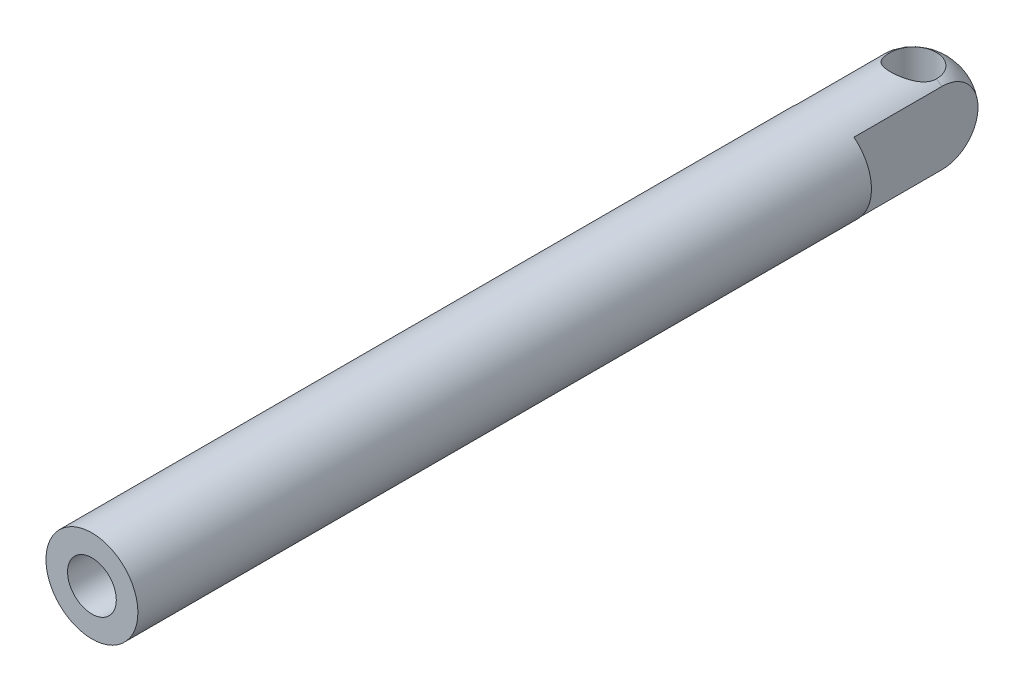
ISO-10303-21;
HEADER;
FILE_DESCRIPTION(('STEP AP214'),'2;1');
FILE_NAME('part.step','',(''),(''),'','','');
FILE_SCHEMA(('AUTOMOTIVE_DESIGN { 1 0 10303 214 1 1 1 1 }'));
ENDSEC;
DATA;
#1=APPLICATION_CONTEXT('core data for automotive mechanical design processes');
#2=APPLICATION_PROTOCOL_DEFINITION('international standard','automotive_design',2000,#1);
#3=PRODUCT_CONTEXT('',#1,'mechanical');
#4=PRODUCT('Part','Part','',(#3));
#5=PRODUCT_RELATED_PRODUCT_CATEGORY('part','',(#4));
#6=PRODUCT_DEFINITION_FORMATION('','',#4);
#7=PRODUCT_DEFINITION_CONTEXT('part definition',#1,'design');
#8=PRODUCT_DEFINITION('design','',#6,#7);
#9=PRODUCT_DEFINITION_SHAPE('','',#8);
#10=(LENGTH_UNIT() NAMED_UNIT(*) SI_UNIT(.MILLI.,.METRE.));
#11=(NAMED_UNIT(*) PLANE_ANGLE_UNIT() SI_UNIT($,.RADIAN.));
#12=(NAMED_UNIT(*) SI_UNIT($,.STERADIAN.) SOLID_ANGLE_UNIT());
#13=UNCERTAINTY_MEASURE_WITH_UNIT(LENGTH_MEASURE(1.E-05),#10,'distance_accuracy_value','');
#14=(GEOMETRIC_REPRESENTATION_CONTEXT(3) GLOBAL_UNCERTAINTY_ASSIGNED_CONTEXT((#13)) GLOBAL_UNIT_ASSIGNED_CONTEXT((#10,
#11,#12)) REPRESENTATION_CONTEXT('',''));
#15=CARTESIAN_POINT('',(0.,0.,0.));
#16=DIRECTION('',(0.,0.,1.));
#17=DIRECTION('',(1.,0.,0.));
#18=AXIS2_PLACEMENT_3D('',#15,#16,#17);
#19=CARTESIAN_POINT('',(0.,0.,1100.));
#20=DIRECTION('',(0.,0.,-1.));
#21=DIRECTION('',(-1.,0.,0.));
#22=AXIS2_PLACEMENT_3D('',#19,#20,#21);
#23=CYLINDRICAL_SURFACE('',#22,115.);
#24=CARTESIAN_POINT('',(0.,0.,1100.));
#25=DIRECTION('',(0.,0.,1.));
#26=DIRECTION('',(1.,0.,0.));
#27=AXIS2_PLACEMENT_3D('',#24,#25,#26);
#28=CIRCLE('',#27,115.);
#29=CARTESIAN_POINT('',(115.,0.,1100.));
#30=VERTEX_POINT('',#29);
#31=EDGE_CURVE('E116',#30,#30,#28,.T.);
#32=ORIENTED_EDGE('',*,*,#31,.F.);
#33=EDGE_LOOP('',(#32));
#34=FACE_BOUND('',#33,.T.);
#35=CARTESIAN_POINT('',(0.,0.,-955.));
#36=DIRECTION('',(0.,0.,-1.));
#37=DIRECTION('',(-1.,0.,0.));
#38=AXIS2_PLACEMENT_3D('',#35,#36,#37);
#39=CIRCLE('',#38,115.);
#40=CARTESIAN_POINT('',(-71.25,90.2686961244041,-955.));
#41=VERTEX_POINT('',#40);
#42=CARTESIAN_POINT('',(-57.5,99.5929214352104,-955.));
#43=VERTEX_POINT('',#42);
#44=EDGE_CURVE('E94',#41,#43,#39,.T.);
#45=ORIENTED_EDGE('',*,*,#44,.F.);
#46=DIRECTION('',(0.,0.,-1.));
#47=VECTOR('',#46,1.);
#48=CARTESIAN_POINT('',(-71.2499999999997,90.2686961244043,1100.));
#49=LINE('',#48,#47);
#50=CARTESIAN_POINT('',(-71.25,90.2686961244041,-735.));
#51=VERTEX_POINT('',#50);
#52=EDGE_CURVE('E64',#41,#51,#49,.F.);
#53=ORIENTED_EDGE('',*,*,#52,.T.);
#54=CARTESIAN_POINT('',(0.,0.,-735.));
#55=DIRECTION('',(0.,0.,1.));
#56=DIRECTION('',(1.,0.,0.));
#57=AXIS2_PLACEMENT_3D('',#54,#55,#56);
#58=CIRCLE('',#57,115.);
#59=CARTESIAN_POINT('',(-71.25,-90.2686961244041,-735.));
#60=VERTEX_POINT('',#59);
#61=EDGE_CURVE('E49',#51,#60,#58,.T.);
#62=ORIENTED_EDGE('',*,*,#61,.T.);
#63=DIRECTION('',(0.,0.,-1.));
#64=VECTOR('',#63,1.);
#65=CARTESIAN_POINT('',(-71.2499999999997,-90.2686961244043,1100.));
#66=LINE('',#65,#64);
#67=CARTESIAN_POINT('',(-71.2499999999997,-90.2686961244043,-955.));
#68=VERTEX_POINT('',#67);
#69=EDGE_CURVE('E108',#60,#68,#66,.T.);
#70=ORIENTED_EDGE('',*,*,#69,.T.);
#71=CARTESIAN_POINT('',(-57.5,-99.5929214352104,-955.));
#72=VERTEX_POINT('',#71);
#73=EDGE_CURVE('E57',#72,#68,#39,.T.);
#74=ORIENTED_EDGE('',*,*,#73,.F.);
#75=CARTESIAN_POINT('',(0.,-115.,-897.5));
#76=CARTESIAN_POINT('',(0.756039926193434,-114.999999631967,-897.500000432809));
#77=CARTESIAN_POINT('',(1.51209474049783,-114.9925400002,-897.514915561743));
#78=CARTESIAN_POINT('',(3.02281407863114,-114.962748266929,-897.57453400003));
#79=CARTESIAN_POINT('',(3.77747843127836,-114.940414442841,-897.619240759561));
#80=CARTESIAN_POINT('',(5.28412678755319,-114.881010387195,-897.7383268216));
#81=CARTESIAN_POINT('',(6.03610984888096,-114.84393540827,-897.812715683214));
#82=CARTESIAN_POINT('',(7.53579035985064,-114.755288294118,-897.990946701532));
#83=CARTESIAN_POINT('',(8.28348735976146,-114.703714664983,-898.094791893359));
#84=CARTESIAN_POINT('',(9.77431659971768,-114.586310667988,-898.331814579295));
#85=CARTESIAN_POINT('',(10.5174397895978,-114.520457961659,-898.46503803896));
#86=CARTESIAN_POINT('',(11.9965952698237,-114.374972804063,-898.760327289052));
#87=CARTESIAN_POINT('',(12.732626832776,-114.295338954809,-898.922396005651));
#88=CARTESIAN_POINT('',(14.9278119005363,-114.036525121805,-899.451152414411));
#89=CARTESIAN_POINT('',(16.374630682964,-113.837387021987,-899.860482083411));
#90=CARTESIAN_POINT('',(19.2192553604664,-113.391738083302,-900.786533039665));
#91=CARTESIAN_POINT('',(20.6172308265571,-113.145415580846,-901.302828021905));
#92=CARTESIAN_POINT('',(23.3621431455185,-112.610679940459,-902.438926815576));
#93=CARTESIAN_POINT('',(24.7090788987355,-112.322265896311,-903.058732855606));
#94=CARTESIAN_POINT('',(27.3444469912767,-111.709942598463,-904.396494277195));
#95=CARTESIAN_POINT('',(28.6328903145282,-111.386040048249,-905.114431128975));
#96=CARTESIAN_POINT('',(31.1454916920329,-110.709761453484,-906.6432915934));
#97=CARTESIAN_POINT('',(32.3696474551825,-110.357384395282,-907.454218516786));
#98=CARTESIAN_POINT('',(34.8203558940024,-109.609679277469,-909.215661471305));
#99=CARTESIAN_POINT('',(36.0425740731368,-109.213042473018,-910.171654104824));
#100=CARTESIAN_POINT('',(38.4031684838954,-108.405503186936,-912.176583704386));
#101=CARTESIAN_POINT('',(39.5415418254895,-107.994600214285,-913.225523871476));
#102=CARTESIAN_POINT('',(41.7300653973575,-107.167956612408,-915.411549309096));
#103=CARTESIAN_POINT('',(42.7801526952142,-106.752212768839,-916.54869636393));
#104=CARTESIAN_POINT('',(44.7862205870241,-105.926254101274,-918.905141627569));
#105=CARTESIAN_POINT('',(45.7421970798222,-105.516039518904,-920.124443412612));
#106=CARTESIAN_POINT('',(47.625340381661,-104.680318438948,-922.737508610054));
#107=CARTESIAN_POINT('',(48.544498522214,-104.256099974802,-924.137466526771));
#108=CARTESIAN_POINT('',(50.2609148362852,-103.43956750798,-927.019604493645));
#109=CARTESIAN_POINT('',(51.0581648876982,-103.047255631889,-928.501790013246));
#110=CARTESIAN_POINT('',(52.1567191513199,-102.493144746503,-930.779400826146));
#111=CARTESIAN_POINT('',(52.5066497716825,-102.31418552947,-931.547570106338));
#112=CARTESIAN_POINT('',(53.1732926756907,-101.969317877728,-933.101026779879));
#113=CARTESIAN_POINT('',(53.490008967781,-101.80340786879,-933.886312093745));
#114=CARTESIAN_POINT('',(54.0893246377893,-101.486254881608,-935.472735887457));
#115=CARTESIAN_POINT('',(54.3719226434949,-101.335012493333,-936.273875003424));
#116=CARTESIAN_POINT('',(54.9020568842566,-101.04877489629,-937.890424944825));
#117=CARTESIAN_POINT('',(55.1495979508498,-100.913777449036,-938.705833786171));
#118=CARTESIAN_POINT('',(55.5950926584644,-100.668994003689,-940.300358924188));
#119=CARTESIAN_POINT('',(55.7951236206591,-100.558184383544,-941.078738099718));
#120=CARTESIAN_POINT('',(56.1627635665738,-100.353317269723,-942.645198713617));
#121=CARTESIAN_POINT('',(56.3303768728474,-100.259257542757,-943.433278843539));
#122=CARTESIAN_POINT('',(56.6326291042369,-100.088837733909,-945.017723949384));
#123=CARTESIAN_POINT('',(56.7672647241471,-100.012479426202,-945.814089747411));
#124=CARTESIAN_POINT('',(57.0030171865704,-99.8782981348512,-947.413225495293));
#125=CARTESIAN_POINT('',(57.1041380984085,-99.8204729009671,-948.215994655528));
#126=CARTESIAN_POINT('',(57.2724234473565,-99.7240137904763,-949.825653897568));
#127=CARTESIAN_POINT('',(57.3396121667856,-99.6853661904514,-950.632540613923));
#128=CARTESIAN_POINT('',(57.439863213353,-99.6276339662686,-952.249030383599));
#129=CARTESIAN_POINT('',(57.4729296704659,-99.6085469746021,-953.058633096288));
#130=CARTESIAN_POINT('',(57.504809509286,-99.5901465279169,-954.678737213077));
#131=CARTESIAN_POINT('',(57.5036235394099,-99.5908326985817,-955.489238599875));
#132=CARTESIAN_POINT('',(57.4670182378401,-99.6119572651791,-957.109131910917));
#133=CARTESIAN_POINT('',(57.4315998689858,-99.6323951055655,-957.918523865724));
#134=CARTESIAN_POINT('',(57.2867443378253,-99.7158050688549,-960.148629469244));
#135=CARTESIAN_POINT('',(57.1415111568199,-99.7992980006931,-961.566461654727));
#136=CARTESIAN_POINT('',(56.74715307412,-100.024054388127,-964.382587204817));
#137=CARTESIAN_POINT('',(56.4980379217935,-100.165312422419,-965.780882390256));
#138=CARTESIAN_POINT('',(55.8987313897626,-100.500993289944,-968.549474129445));
#139=CARTESIAN_POINT('',(55.5485146876636,-100.695429441789,-969.919763576555));
#140=CARTESIAN_POINT('',(54.7506543690294,-101.131460009223,-972.623950185859));
#141=CARTESIAN_POINT('',(54.3030055628721,-101.373056936711,-973.957845405292));
#142=CARTESIAN_POINT('',(53.3028640421449,-101.902561337218,-976.612807639544));
#143=CARTESIAN_POINT('',(52.7481799858778,-102.191413138314,-977.932859168227));
#144=CARTESIAN_POINT('',(51.5455433044256,-102.803267968911,-980.521441799243));
#145=CARTESIAN_POINT('',(50.8975906337853,-103.126271015054,-981.789972876468));
#146=CARTESIAN_POINT('',(49.5125582915078,-103.798357758824,-984.270726308318));
#147=CARTESIAN_POINT('',(48.7754481390498,-104.147450360174,-985.482929208521));
#148=CARTESIAN_POINT('',(47.2164488041148,-104.863448210345,-987.846019316552));
#149=CARTESIAN_POINT('',(46.3945539489378,-105.230354650168,-988.996902413826));
#150=CARTESIAN_POINT('',(44.5604896200246,-106.021140402594,-991.375052976015));
#151=CARTESIAN_POINT('',(43.5374093623827,-106.446341862118,-992.593485064299));
#152=CARTESIAN_POINT('',(41.3940851145652,-107.297994310601,-994.94128936598));
#153=CARTESIAN_POINT('',(40.2738339511412,-107.724445389559,-996.070654992638));
#154=CARTESIAN_POINT('',(37.9411110892785,-108.568001016734,-998.234874912984));
#155=CARTESIAN_POINT('',(36.7285966602381,-108.985101116957,-999.269684920083));
#156=CARTESIAN_POINT('',(34.2176012597706,-109.799352171425,-1001.23797774279));
#157=CARTESIAN_POINT('',(32.9191196677261,-110.196502981613,-1002.17145982675));
#158=CARTESIAN_POINT('',(30.180184047429,-110.978726236119,-1003.97157632688));
#159=CARTESIAN_POINT('',(28.7359340199946,-111.362373826484,-1004.83306989169));
#160=CARTESIAN_POINT('',(25.7687974093903,-112.086130871539,-1006.4301230848));
#161=CARTESIAN_POINT('',(24.2459071685366,-112.426238298542,-1007.16567684854));
#162=CARTESIAN_POINT('',(21.1327463003638,-113.052758086648,-1008.50256724992));
#163=CARTESIAN_POINT('',(19.5425192850707,-113.339204569421,-1009.10398922533));
#164=CARTESIAN_POINT('',(16.3059802117296,-113.849890864604,-1010.16579197716));
#165=CARTESIAN_POINT('',(14.659674629808,-114.074137832845,-1010.62618897864));
#166=CARTESIAN_POINT('',(11.4632047192093,-114.437600072419,-1011.36762870229));
#167=CARTESIAN_POINT('',(9.91637286310852,-114.582320238039,-1011.66036914825));
#168=CARTESIAN_POINT('',(6.79940917810755,-114.809446464326,-1012.11828715779));
#169=CARTESIAN_POINT('',(5.22927862129342,-114.891855914424,-1012.28347165986));
#170=CARTESIAN_POINT('',(2.07932335511353,-114.99199375301,-1012.48405134883));
#171=CARTESIAN_POINT('',(0.499502774961316,-115.009748002694,-1012.51949842896));
#172=CARTESIAN_POINT('',(-2.65704791013921,-114.980132207341,-1012.46026065505));
#173=CARTESIAN_POINT('',(-4.23377814876672,-114.932765044441,-1012.36558156011));
#174=CARTESIAN_POINT('',(-7.24900068560403,-114.780448517955,-1012.05976820056));
#175=CARTESIAN_POINT('',(-8.68872217543315,-114.680254828179,-1011.8582451553));
#176=CARTESIAN_POINT('',(-11.5442945106091,-114.428071157171,-1011.34787232871));
#177=CARTESIAN_POINT('',(-12.9601468857035,-114.276084508642,-1011.03902945303));
#178=CARTESIAN_POINT('',(-15.7589346501385,-113.923859304687,-1010.31722028618));
#179=CARTESIAN_POINT('',(-17.1418682040933,-113.723618065721,-1009.90424820412));
#180=CARTESIAN_POINT('',(-19.86654595913,-113.279415572935,-1008.97815295026));
#181=CARTESIAN_POINT('',(-21.2082884268221,-113.035452482172,-1008.46502557044));
#182=CARTESIAN_POINT('',(-23.880897489362,-112.5016105184,-1007.32706764311));
#183=CARTESIAN_POINT('',(-25.2103616515162,-112.210620237904,-1006.69946785276));
#184=CARTESIAN_POINT('',(-27.8111662225543,-111.59446813568,-1005.34815623474));
#185=CARTESIAN_POINT('',(-29.082506120613,-111.269306013714,-1004.62444356261));
#186=CARTESIAN_POINT('',(-31.5616183205955,-110.591664351637,-1003.0857921916));
#187=CARTESIAN_POINT('',(-32.7693696687149,-110.239175900343,-1002.27082369515));
#188=CARTESIAN_POINT('',(-35.1158123979574,-109.514327042851,-1000.55483038709));
#189=CARTESIAN_POINT('',(-36.2544999782216,-109.141965545075,-999.653800846205));
#190=CARTESIAN_POINT('',(-38.5665301149181,-108.347865372805,-997.677944661801));
#191=CARTESIAN_POINT('',(-39.7322855784827,-107.924869834846,-996.594740149521));
#192=CARTESIAN_POINT('',(-41.9695388226546,-107.074692698471,-994.336167972647));
#193=CARTESIAN_POINT('',(-43.0410307794307,-106.647510843224,-993.160794622108));
#194=CARTESIAN_POINT('',(-44.5734979250476,-106.011838231184,-991.332993713112));
#195=CARTESIAN_POINT('',(-45.0720701748748,-105.800701644033,-990.712636948676));
#196=CARTESIAN_POINT('',(-46.04350748944,-105.381569171776,-989.451110862577));
#197=CARTESIAN_POINT('',(-46.5163747063028,-105.173573024797,-988.809943290476));
#198=CARTESIAN_POINT('',(-47.4356642828128,-104.762165642518,-987.507583576832));
#199=CARTESIAN_POINT('',(-47.8820891385812,-104.558753975576,-986.846393334334));
#200=CARTESIAN_POINT('',(-48.7479330302106,-104.157893217983,-985.504539423803));
#201=CARTESIAN_POINT('',(-49.1673432718118,-103.960446080004,-984.823869517525));
#202=CARTESIAN_POINT('',(-50.4230543067088,-103.360550292388,-982.687193445124));
#203=CARTESIAN_POINT('',(-51.2121770973233,-102.970727111135,-981.199460793565));
#204=CARTESIAN_POINT('',(-52.6604836742353,-102.237631258297,-978.151023950491));
#205=CARTESIAN_POINT('',(-53.3196816844298,-101.894353492302,-976.590327770044));
#206=CARTESIAN_POINT('',(-54.2051804569244,-101.424403053757,-974.203349911754));
#207=CARTESIAN_POINT('',(-54.4830649598738,-101.275283870952,-973.400273678963));
#208=CARTESIAN_POINT('',(-55.0036483734081,-100.993496724154,-971.780112954271));
#209=CARTESIAN_POINT('',(-55.2463563693533,-100.860824513534,-970.963032140649));
#210=CARTESIAN_POINT('',(-55.6957760306153,-100.613350653786,-969.316387578991));
#211=CARTESIAN_POINT('',(-55.9024885524288,-100.498548579451,-968.486824128485));
#212=CARTESIAN_POINT('',(-56.2791501611203,-100.288104202955,-966.816929259857));
#213=CARTESIAN_POINT('',(-56.4490977748551,-100.192462668553,-965.976597411681));
#214=CARTESIAN_POINT('',(-56.736992902327,-100.029686864408,-964.368319865377));
#215=CARTESIAN_POINT('',(-56.8583669988458,-99.9606969052523,-963.601173319719));
#216=CARTESIAN_POINT('',(-57.070067628939,-99.8399832319084,-962.061258907232));
#217=CARTESIAN_POINT('',(-57.1603946750298,-99.7882592326992,-961.288491133412));
#218=CARTESIAN_POINT('',(-57.3096654456911,-99.7026060629048,-959.738989810187));
#219=CARTESIAN_POINT('',(-57.3686109205854,-99.6686758998606,-958.962256484403));
#220=CARTESIAN_POINT('',(-57.454904088652,-99.6189564332258,-957.406448322968));
#221=CARTESIAN_POINT('',(-57.4822515239774,-99.6031672776699,-956.627373468262));
#222=CARTESIAN_POINT('',(-57.5052371157365,-99.589898506077,-955.068933240547));
#223=CARTESIAN_POINT('',(-57.5008888683154,-99.5924110393675,-954.289568135489));
#224=CARTESIAN_POINT('',(-57.4605309260017,-99.615701142035,-952.731848495079));
#225=CARTESIAN_POINT('',(-57.4245176841276,-99.6364807576149,-951.953494082725));
#226=CARTESIAN_POINT('',(-57.3209665603307,-99.6960902023079,-950.399686608433));
#227=CARTESIAN_POINT('',(-57.2534334295366,-99.7349173110409,-949.624233126978));
#228=CARTESIAN_POINT('',(-57.0871056332497,-99.8302127262599,-948.077753745496));
#229=CARTESIAN_POINT('',(-56.9883079687483,-99.88668272511,-947.306728277448));
#230=CARTESIAN_POINT('',(-56.6673584968348,-100.069317044624,-945.149537369074));
#231=CARTESIAN_POINT('',(-56.410056996097,-100.214915854682,-943.770043780577));
#232=CARTESIAN_POINT('',(-55.7971757470509,-100.557435130884,-941.039939943489));
#233=CARTESIAN_POINT('',(-55.4416038290174,-100.75435150793,-939.689327402863));
#234=CARTESIAN_POINT('',(-54.635622638641,-101.193672037181,-937.023975355456));
#235=CARTESIAN_POINT('',(-54.1851912494906,-101.436086796053,-935.709244295455));
#236=CARTESIAN_POINT('',(-53.1934565263105,-101.959650626916,-933.122491205063));
#237=CARTESIAN_POINT('',(-52.652147181976,-102.240802260589,-931.850472006147));
#238=CARTESIAN_POINT('',(-51.4434079175519,-102.854583657747,-929.270862259647));
#239=CARTESIAN_POINT('',(-50.7699503776319,-103.189402290082,-927.966617402513));
#240=CARTESIAN_POINT('',(-49.3289391664945,-103.885976043569,-925.418788082898));
#241=CARTESIAN_POINT('',(-48.5613827724136,-104.247731944064,-924.175205377207));
#242=CARTESIAN_POINT('',(-46.9363907051099,-104.989394926069,-921.753152991897));
#243=CARTESIAN_POINT('',(-46.0789170228177,-105.369309646293,-920.574711172128));
#244=CARTESIAN_POINT('',(-44.2786768209794,-106.138385804183,-918.288060636244));
#245=CARTESIAN_POINT('',(-43.3359053699268,-106.52754777552,-917.179855987211));
#246=CARTESIAN_POINT('',(-41.2495738637216,-107.353992236728,-914.907834796143));
#247=CARTESIAN_POINT('',(-40.0955388897124,-107.791370788718,-913.75364709984));
#248=CARTESIAN_POINT('',(-37.6912537470597,-108.655423808158,-911.54561564665));
#249=CARTESIAN_POINT('',(-36.4409953740853,-109.082097358743,-910.491780463334));
#250=CARTESIAN_POINT('',(-33.8498872386978,-109.913774342929,-908.490683738797));
#251=CARTESIAN_POINT('',(-32.5089843692621,-110.318764819417,-907.543485555768));
#252=CARTESIAN_POINT('',(-29.7440808072623,-111.09613051583,-905.763412951452));
#253=CARTESIAN_POINT('',(-28.320084909544,-111.4685076146,-904.930531942821));
#254=CARTESIAN_POINT('',(-26.1232440513399,-111.996205177372,-903.769936298879));
#255=CARTESIAN_POINT('',(-25.3779570185928,-112.167534384552,-903.396646811582));
#256=CARTESIAN_POINT('',(-23.8696910734563,-112.498148703657,-902.681896513355));
#257=CARTESIAN_POINT('',(-23.1067141645341,-112.65743517086,-902.34043211985));
#258=CARTESIAN_POINT('',(-21.5641379346627,-112.962854193443,-901.690162046069));
#259=CARTESIAN_POINT('',(-20.7845340924405,-113.108983113067,-901.381365388595));
#260=CARTESIAN_POINT('',(-19.2104018054201,-113.386944229012,-900.797462745457));
#261=CARTESIAN_POINT('',(-18.4158751769259,-113.518778152167,-900.52235268994));
#262=CARTESIAN_POINT('',(-16.8152520483828,-113.766874008643,-900.007250953597));
#263=CARTESIAN_POINT('',(-16.0091876147387,-113.883172285347,-899.767177184207));
#264=CARTESIAN_POINT('',(-14.3853796211442,-114.099656635082,-899.322181835947));
#265=CARTESIAN_POINT('',(-13.5676375510337,-114.199844743814,-899.11725581555));
#266=CARTESIAN_POINT('',(-11.9225041939606,-114.383296966167,-898.74331011255));
#267=CARTESIAN_POINT('',(-11.0951175049056,-114.466568821348,-898.574274003672));
#268=CARTESIAN_POINT('',(-9.43227655563561,-114.615569489628,-898.272616922289));
#269=CARTESIAN_POINT('',(-8.59682357872582,-114.681301047154,-898.139990252923));
#270=CARTESIAN_POINT('',(-7.11657618506717,-114.78139287965,-897.938420570041));
#271=CARTESIAN_POINT('',(-6.47306173023466,-114.819495250392,-897.861836569897));
#272=CARTESIAN_POINT('',(-5.18343427575204,-114.884936794181,-897.730444717982));
#273=CARTESIAN_POINT('',(-4.53732203061077,-114.912278892345,-897.675630948065));
#274=CARTESIAN_POINT('',(-3.24322242753817,-114.956081540322,-897.587874735845));
#275=CARTESIAN_POINT('',(-2.59523500121499,-114.972541688093,-897.554933101627));
#276=CARTESIAN_POINT('',(-1.2981688664785,-114.994502486418,-897.510992723836));
#277=CARTESIAN_POINT('',(-0.649089920174928,-115.000000315971,-897.499999628416));
#278=CARTESIAN_POINT('',(0.,-115.,-897.5));
#279=B_SPLINE_CURVE_WITH_KNOTS('',3,(#75,#76,#77,#78,#79,#80,#81,#82,#83,#84,#85,#86,#87,#88,
#89,#90,#91,#92,#93,#94,#95,#96,#97,#98,#99,#100,#101,#102,#103,#104,#105,#106,#107,#108,#109,
#110,#111,#112,#113,#114,#115,#116,#117,#118,#119,#120,#121,#122,#123,#124,#125,#126,#127,#128,
#129,#130,#131,#132,#133,#134,#135,#136,#137,#138,#139,#140,#141,#142,#143,#144,#145,#146,#147,
#148,#149,#150,#151,#152,#153,#154,#155,#156,#157,#158,#159,#160,#161,#162,#163,#164,#165,#166,
#167,#168,#169,#170,#171,#172,#173,#174,#175,#176,#177,#178,#179,#180,#181,#182,#183,#184,#185,
#186,#187,#188,#189,#190,#191,#192,#193,#194,#195,#196,#197,#198,#199,#200,#201,#202,#203,#204,
#205,#206,#207,#208,#209,#210,#211,#212,#213,#214,#215,#216,#217,#218,#219,#220,#221,#222,#223,
#224,#225,#226,#227,#228,#229,#230,#231,#232,#233,#234,#235,#236,#237,#238,#239,#240,#241,#242,
#243,#244,#245,#246,#247,#248,#249,#250,#251,#252,#253,#254,#255,#256,#257,#258,#259,#260,#261,
#262,#263,#264,#265,#266,#267,#268,#269,#270,#271,#272,#273,#274,#275,#276,#277,#278),
.UNSPECIFIED.,.T.,.F.,(4,2,2,2,2,2,2,2,2,2,2,2,2,2,2,2,2,2,2,2,2,2,2,2,2,2,2,2,2,2,2,2,2,2,2,2,
2,2,2,2,2,2,2,2,2,2,2,2,2,2,2,2,2,2,2,2,2,2,2,2,2,2,2,2,2,2,2,2,2,2,2,2,2,2,2,2,2,2,2,2,2,2,2,2,
2,2,2,2,2,2,2,2,2,2,2,2,2,2,2,2,2,4),(0.,2.26796186538117,4.53618642977221,6.80514206504901,
9.07433157407714,11.3470969952568,13.6200931056915,18.1643392217283,22.690811339866,
27.2173809257509,31.743096949385,36.2689741528251,41.0686294571016,45.868450122351,
50.6716637084774,55.4750865161896,60.6516986802541,65.8286555850784,68.4165500538143,
71.0041318442833,73.5918176707376,76.1791465152906,78.6121137539573,81.0447563580191,
83.4776426752703,85.9102334853916,88.3410810263639,90.7716343161315,93.2021415942568,
95.6325805125806,99.9100790173004,104.187176167241,108.465345510923,112.743742782737,
117.121394063054,121.499047476859,125.878201758911,130.257649227819,135.192750717524,
140.128216831658,145.065982824372,150.003784467868,155.171643941223,160.339743996977,
165.504546547233,170.66875465884,175.405186128869,180.141359939056,184.875639136277,
189.609708811057,193.976264397034,198.34253906276,202.709056602209,207.075757640839,
211.567041565778,216.05836495479,220.551159186474,225.044200450882,229.978685915811,
234.913476031596,237.383139423159,239.852595725492,242.321818541936,244.791841161358,
249.97042246631,255.148436515569,257.735948812545,260.322791613377,262.909572852992,
265.496457723853,267.834893379732,270.173290431483,272.511557044228,274.8498427376,
277.187125461568,279.52467003162,281.861862367229,284.199278962872,288.426550782891,
292.653485867178,296.881407568967,301.10960899883,305.621690891003,310.13390337652,
314.648030974069,319.162419723726,324.225857693403,329.289727868161,334.35659102903,
339.423162097425,341.975363744668,344.527277740755,347.079894743273,349.632203045852,
352.178431935037,354.724338826634,357.269077970932,359.813418721247,361.760509790648,
363.707071188623,365.653704499864,367.600838685716),.UNSPECIFIED.);
#280=CARTESIAN_POINT('',(57.5,-99.5929214352104,-955.));
#281=VERTEX_POINT('',#280);
#282=EDGE_CURVE('E124',#72,#281,#279,.T.);
#283=ORIENTED_EDGE('',*,*,#282,.T.);
#284=CARTESIAN_POINT('',(71.25,-90.2686961244041,-955.));
#285=VERTEX_POINT('',#284);
#286=EDGE_CURVE('E264',#285,#281,#39,.T.);
#287=ORIENTED_EDGE('',*,*,#286,.F.);
#288=DIRECTION('',(0.,0.,-1.));
#289=VECTOR('',#288,1.);
#290=CARTESIAN_POINT('',(71.2499999999997,-90.2686961244043,1100.));
#291=LINE('',#290,#289);
#292=CARTESIAN_POINT('',(71.25,-90.2686961244044,-735.));
#293=VERTEX_POINT('',#292);
#294=EDGE_CURVE('E111',#285,#293,#291,.F.);
#295=ORIENTED_EDGE('',*,*,#294,.T.);
#296=CARTESIAN_POINT('',(0.,0.,-735.));
#297=DIRECTION('',(0.,0.,1.));
#298=DIRECTION('',(1.,0.,0.));
#299=AXIS2_PLACEMENT_3D('',#296,#297,#298);
#300=CIRCLE('',#299,115.);
#301=CARTESIAN_POINT('',(71.25,90.2686961244044,-735.));
#302=VERTEX_POINT('',#301);
#303=EDGE_CURVE('E123',#293,#302,#300,.T.);
#304=ORIENTED_EDGE('',*,*,#303,.T.);
#305=DIRECTION('',(0.,0.,-1.));
#306=VECTOR('',#305,1.);
#307=CARTESIAN_POINT('',(71.2499999999997,90.2686961244043,1100.));
#308=LINE('',#307,#306);
#309=CARTESIAN_POINT('',(71.25,90.2686961244041,-955.));
#310=VERTEX_POINT('',#309);
#311=EDGE_CURVE('E109',#302,#310,#308,.T.);
#312=ORIENTED_EDGE('',*,*,#311,.T.);
#313=CARTESIAN_POINT('',(57.5,99.5929214352104,-955.));
#314=VERTEX_POINT('',#313);
#315=EDGE_CURVE('E103',#314,#310,#39,.T.);
#316=ORIENTED_EDGE('',*,*,#315,.F.);
#317=CARTESIAN_POINT('',(0.,115.,-897.5));
#318=CARTESIAN_POINT('',(-0.756039926193434,114.999999631967,-897.500000432809));
#319=CARTESIAN_POINT('',(-1.51209474049783,114.9925400002,-897.514915561743));
#320=CARTESIAN_POINT('',(-3.02281407863114,114.962748266929,-897.57453400003));
#321=CARTESIAN_POINT('',(-3.77747843127836,114.940414442841,-897.619240759561));
#322=CARTESIAN_POINT('',(-5.28412678755319,114.881010387195,-897.7383268216));
#323=CARTESIAN_POINT('',(-6.03610984888096,114.84393540827,-897.812715683214));
#324=CARTESIAN_POINT('',(-7.53579035985064,114.755288294118,-897.990946701532));
#325=CARTESIAN_POINT('',(-8.28348735976146,114.703714664983,-898.094791893359));
#326=CARTESIAN_POINT('',(-9.77431659971768,114.586310667988,-898.331814579295));
#327=CARTESIAN_POINT('',(-10.5174397895978,114.520457961659,-898.46503803896));
#328=CARTESIAN_POINT('',(-11.9965952698237,114.374972804063,-898.760327289052));
#329=CARTESIAN_POINT('',(-12.732626832776,114.295338954809,-898.922396005651));
#330=CARTESIAN_POINT('',(-14.9278119005363,114.036525121805,-899.451152414411));
#331=CARTESIAN_POINT('',(-16.374630682964,113.837387021987,-899.860482083411));
#332=CARTESIAN_POINT('',(-19.2192553604664,113.391738083302,-900.786533039665));
#333=CARTESIAN_POINT('',(-20.6172308265571,113.145415580846,-901.302828021905));
#334=CARTESIAN_POINT('',(-23.3621431455185,112.610679940459,-902.438926815576));
#335=CARTESIAN_POINT('',(-24.7090788987355,112.322265896311,-903.058732855606));
#336=CARTESIAN_POINT('',(-27.3444469912767,111.709942598463,-904.396494277195));
#337=CARTESIAN_POINT('',(-28.6328903145282,111.386040048249,-905.114431128975));
#338=CARTESIAN_POINT('',(-31.1454916920329,110.709761453484,-906.6432915934));
#339=CARTESIAN_POINT('',(-32.3696474551825,110.357384395282,-907.454218516786));
#340=CARTESIAN_POINT('',(-34.8203558940024,109.609679277469,-909.215661471305));
#341=CARTESIAN_POINT('',(-36.0425740731368,109.213042473018,-910.171654104824));
#342=CARTESIAN_POINT('',(-38.4031684838954,108.405503186936,-912.176583704386));
#343=CARTESIAN_POINT('',(-39.5415418254895,107.994600214285,-913.225523871476));
#344=CARTESIAN_POINT('',(-41.7300653973575,107.167956612408,-915.411549309096));
#345=CARTESIAN_POINT('',(-42.7801526952142,106.752212768839,-916.54869636393));
#346=CARTESIAN_POINT('',(-44.7862205870241,105.926254101274,-918.905141627569));
#347=CARTESIAN_POINT('',(-45.7421970798222,105.516039518904,-920.124443412612));
#348=CARTESIAN_POINT('',(-47.625340381661,104.680318438948,-922.737508610054));
#349=CARTESIAN_POINT('',(-48.544498522214,104.256099974802,-924.137466526771));
#350=CARTESIAN_POINT('',(-50.2609148362852,103.43956750798,-927.019604493645));
#351=CARTESIAN_POINT('',(-51.0581648876982,103.047255631889,-928.501790013246));
#352=CARTESIAN_POINT('',(-52.1567191513199,102.493144746503,-930.779400826146));
#353=CARTESIAN_POINT('',(-52.5066497716825,102.31418552947,-931.547570106338));
#354=CARTESIAN_POINT('',(-53.1732926756907,101.969317877728,-933.101026779879));
#355=CARTESIAN_POINT('',(-53.490008967781,101.80340786879,-933.886312093745));
#356=CARTESIAN_POINT('',(-54.0893246377893,101.486254881608,-935.472735887457));
#357=CARTESIAN_POINT('',(-54.3719226434949,101.335012493333,-936.273875003424));
#358=CARTESIAN_POINT('',(-54.9020568842566,101.04877489629,-937.890424944825));
#359=CARTESIAN_POINT('',(-55.1495979508498,100.913777449036,-938.705833786171));
#360=CARTESIAN_POINT('',(-55.5950926584644,100.668994003689,-940.300358924188));
#361=CARTESIAN_POINT('',(-55.7951236206591,100.558184383544,-941.078738099718));
#362=CARTESIAN_POINT('',(-56.1627635665738,100.353317269723,-942.645198713617));
#363=CARTESIAN_POINT('',(-56.3303768728474,100.259257542757,-943.433278843539));
#364=CARTESIAN_POINT('',(-56.6326291042369,100.088837733909,-945.017723949384));
#365=CARTESIAN_POINT('',(-56.7672647241471,100.012479426202,-945.814089747411));
#366=CARTESIAN_POINT('',(-57.0030171865704,99.8782981348512,-947.413225495293));
#367=CARTESIAN_POINT('',(-57.1041380984085,99.8204729009671,-948.215994655528));
#368=CARTESIAN_POINT('',(-57.2724234473565,99.7240137904763,-949.825653897568));
#369=CARTESIAN_POINT('',(-57.3396121667856,99.6853661904514,-950.632540613923));
#370=CARTESIAN_POINT('',(-57.439863213353,99.6276339662686,-952.249030383599));
#371=CARTESIAN_POINT('',(-57.4729296704659,99.6085469746021,-953.058633096288));
#372=CARTESIAN_POINT('',(-57.504809509286,99.5901465279169,-954.678737213077));
#373=CARTESIAN_POINT('',(-57.5036235394099,99.5908326985817,-955.489238599875));
#374=CARTESIAN_POINT('',(-57.4670182378401,99.6119572651791,-957.109131910917));
#375=CARTESIAN_POINT('',(-57.4315998689858,99.6323951055655,-957.918523865724));
#376=CARTESIAN_POINT('',(-57.2867443378253,99.7158050688549,-960.148629469244));
#377=CARTESIAN_POINT('',(-57.1415111568199,99.7992980006931,-961.566461654727));
#378=CARTESIAN_POINT('',(-56.74715307412,100.024054388127,-964.382587204817));
#379=CARTESIAN_POINT('',(-56.4980379217935,100.165312422419,-965.780882390256));
#380=CARTESIAN_POINT('',(-55.8987313897626,100.500993289944,-968.549474129445));
#381=CARTESIAN_POINT('',(-55.5485146876636,100.695429441789,-969.919763576555));
#382=CARTESIAN_POINT('',(-54.7506543690294,101.131460009223,-972.623950185859));
#383=CARTESIAN_POINT('',(-54.3030055628721,101.373056936711,-973.957845405292));
#384=CARTESIAN_POINT('',(-53.3028640421449,101.902561337218,-976.612807639544));
#385=CARTESIAN_POINT('',(-52.7481799858778,102.191413138314,-977.932859168227));
#386=CARTESIAN_POINT('',(-51.5455433044256,102.803267968911,-980.521441799243));
#387=CARTESIAN_POINT('',(-50.8975906337853,103.126271015054,-981.789972876468));
#388=CARTESIAN_POINT('',(-49.5125582915078,103.798357758824,-984.270726308318));
#389=CARTESIAN_POINT('',(-48.7754481390498,104.147450360174,-985.482929208521));
#390=CARTESIAN_POINT('',(-47.2164488041148,104.863448210345,-987.846019316552));
#391=CARTESIAN_POINT('',(-46.3945539489378,105.230354650168,-988.996902413826));
#392=CARTESIAN_POINT('',(-44.5604896200246,106.021140402594,-991.375052976015));
#393=CARTESIAN_POINT('',(-43.5374093623827,106.446341862118,-992.593485064299));
#394=CARTESIAN_POINT('',(-41.3940851145652,107.297994310601,-994.94128936598));
#395=CARTESIAN_POINT('',(-40.2738339511412,107.724445389559,-996.070654992638));
#396=CARTESIAN_POINT('',(-37.9411110892785,108.568001016734,-998.234874912984));
#397=CARTESIAN_POINT('',(-36.7285966602381,108.985101116957,-999.269684920083));
#398=CARTESIAN_POINT('',(-34.2176012597706,109.799352171425,-1001.23797774279));
#399=CARTESIAN_POINT('',(-32.9191196677261,110.196502981613,-1002.17145982675));
#400=CARTESIAN_POINT('',(-30.180184047429,110.978726236119,-1003.97157632688));
#401=CARTESIAN_POINT('',(-28.7359340199946,111.362373826484,-1004.83306989169));
#402=CARTESIAN_POINT('',(-25.7687974093903,112.086130871539,-1006.4301230848));
#403=CARTESIAN_POINT('',(-24.2459071685366,112.426238298542,-1007.16567684854));
#404=CARTESIAN_POINT('',(-21.1327463003638,113.052758086648,-1008.50256724992));
#405=CARTESIAN_POINT('',(-19.5425192850707,113.339204569421,-1009.10398922533));
#406=CARTESIAN_POINT('',(-16.3059802117296,113.849890864604,-1010.16579197716));
#407=CARTESIAN_POINT('',(-14.659674629808,114.074137832845,-1010.62618897864));
#408=CARTESIAN_POINT('',(-11.4632047192093,114.437600072419,-1011.36762870229));
#409=CARTESIAN_POINT('',(-9.91637286310852,114.582320238039,-1011.66036914825));
#410=CARTESIAN_POINT('',(-6.79940917810755,114.809446464326,-1012.11828715779));
#411=CARTESIAN_POINT('',(-5.22927862129342,114.891855914424,-1012.28347165986));
#412=CARTESIAN_POINT('',(-2.07932335511353,114.99199375301,-1012.48405134883));
#413=CARTESIAN_POINT('',(-0.499502774961316,115.009748002694,-1012.51949842896));
#414=CARTESIAN_POINT('',(2.65704791013921,114.980132207341,-1012.46026065505));
#415=CARTESIAN_POINT('',(4.23377814876672,114.932765044441,-1012.36558156011));
#416=CARTESIAN_POINT('',(7.24900068560403,114.780448517955,-1012.05976820056));
#417=CARTESIAN_POINT('',(8.68872217543315,114.680254828179,-1011.8582451553));
#418=CARTESIAN_POINT('',(11.5442945106091,114.428071157171,-1011.34787232871));
#419=CARTESIAN_POINT('',(12.9601468857035,114.276084508642,-1011.03902945303));
#420=CARTESIAN_POINT('',(15.7589346501385,113.923859304687,-1010.31722028618));
#421=CARTESIAN_POINT('',(17.1418682040933,113.723618065721,-1009.90424820412));
#422=CARTESIAN_POINT('',(19.86654595913,113.279415572935,-1008.97815295026));
#423=CARTESIAN_POINT('',(21.2082884268221,113.035452482172,-1008.46502557044));
#424=CARTESIAN_POINT('',(23.880897489362,112.5016105184,-1007.32706764311));
#425=CARTESIAN_POINT('',(25.2103616515162,112.210620237904,-1006.69946785276));
#426=CARTESIAN_POINT('',(27.8111662225543,111.59446813568,-1005.34815623474));
#427=CARTESIAN_POINT('',(29.082506120613,111.269306013714,-1004.62444356261));
#428=CARTESIAN_POINT('',(31.5616183205955,110.591664351637,-1003.0857921916));
#429=CARTESIAN_POINT('',(32.7693696687149,110.239175900343,-1002.27082369515));
#430=CARTESIAN_POINT('',(35.1158123979574,109.514327042851,-1000.55483038709));
#431=CARTESIAN_POINT('',(36.2544999782216,109.141965545075,-999.653800846205));
#432=CARTESIAN_POINT('',(38.5665301149181,108.347865372805,-997.677944661801));
#433=CARTESIAN_POINT('',(39.7322855784827,107.924869834846,-996.594740149521));
#434=CARTESIAN_POINT('',(41.9695388226546,107.074692698471,-994.336167972647));
#435=CARTESIAN_POINT('',(43.0410307794307,106.647510843224,-993.160794622108));
#436=CARTESIAN_POINT('',(44.5734979250476,106.011838231184,-991.332993713112));
#437=CARTESIAN_POINT('',(45.0720701748748,105.800701644033,-990.712636948676));
#438=CARTESIAN_POINT('',(46.04350748944,105.381569171776,-989.451110862577));
#439=CARTESIAN_POINT('',(46.5163747063028,105.173573024797,-988.809943290476));
#440=CARTESIAN_POINT('',(47.4356642828128,104.762165642518,-987.507583576832));
#441=CARTESIAN_POINT('',(47.8820891385812,104.558753975576,-986.846393334334));
#442=CARTESIAN_POINT('',(48.7479330302106,104.157893217983,-985.504539423803));
#443=CARTESIAN_POINT('',(49.1673432718118,103.960446080004,-984.823869517525));
#444=CARTESIAN_POINT('',(50.4230543067088,103.360550292388,-982.687193445124));
#445=CARTESIAN_POINT('',(51.2121770973233,102.970727111135,-981.199460793565));
#446=CARTESIAN_POINT('',(52.6604836742353,102.237631258297,-978.151023950491));
#447=CARTESIAN_POINT('',(53.3196816844298,101.894353492302,-976.590327770044));
#448=CARTESIAN_POINT('',(54.2051804569244,101.424403053757,-974.203349911754));
#449=CARTESIAN_POINT('',(54.4830649598738,101.275283870952,-973.400273678963));
#450=CARTESIAN_POINT('',(55.0036483734081,100.993496724154,-971.780112954271));
#451=CARTESIAN_POINT('',(55.2463563693533,100.860824513534,-970.963032140649));
#452=CARTESIAN_POINT('',(55.6957760306153,100.613350653786,-969.316387578991));
#453=CARTESIAN_POINT('',(55.9024885524288,100.498548579451,-968.486824128485));
#454=CARTESIAN_POINT('',(56.2791501611203,100.288104202955,-966.816929259857));
#455=CARTESIAN_POINT('',(56.4490977748551,100.192462668553,-965.976597411681));
#456=CARTESIAN_POINT('',(56.736992902327,100.029686864408,-964.368319865377));
#457=CARTESIAN_POINT('',(56.8583669988458,99.9606969052523,-963.601173319719));
#458=CARTESIAN_POINT('',(57.070067628939,99.8399832319084,-962.061258907232));
#459=CARTESIAN_POINT('',(57.1603946750298,99.7882592326992,-961.288491133412));
#460=CARTESIAN_POINT('',(57.3096654456911,99.7026060629048,-959.738989810187));
#461=CARTESIAN_POINT('',(57.3686109205854,99.6686758998606,-958.962256484403));
#462=CARTESIAN_POINT('',(57.454904088652,99.6189564332258,-957.406448322968));
#463=CARTESIAN_POINT('',(57.4822515239774,99.6031672776699,-956.627373468262));
#464=CARTESIAN_POINT('',(57.5052371157365,99.589898506077,-955.068933240547));
#465=CARTESIAN_POINT('',(57.5008888683154,99.5924110393675,-954.289568135489));
#466=CARTESIAN_POINT('',(57.4605309260017,99.615701142035,-952.731848495079));
#467=CARTESIAN_POINT('',(57.4245176841276,99.6364807576149,-951.953494082725));
#468=CARTESIAN_POINT('',(57.3209665603307,99.6960902023079,-950.399686608433));
#469=CARTESIAN_POINT('',(57.2534334295366,99.7349173110409,-949.624233126978));
#470=CARTESIAN_POINT('',(57.0871056332497,99.8302127262599,-948.077753745496));
#471=CARTESIAN_POINT('',(56.9883079687483,99.88668272511,-947.306728277448));
#472=CARTESIAN_POINT('',(56.6673584968348,100.069317044624,-945.149537369074));
#473=CARTESIAN_POINT('',(56.410056996097,100.214915854682,-943.770043780577));
#474=CARTESIAN_POINT('',(55.7971757470509,100.557435130884,-941.039939943489));
#475=CARTESIAN_POINT('',(55.4416038290174,100.75435150793,-939.689327402863));
#476=CARTESIAN_POINT('',(54.635622638641,101.193672037181,-937.023975355456));
#477=CARTESIAN_POINT('',(54.1851912494906,101.436086796053,-935.709244295455));
#478=CARTESIAN_POINT('',(53.1934565263105,101.959650626916,-933.122491205063));
#479=CARTESIAN_POINT('',(52.652147181976,102.240802260589,-931.850472006147));
#480=CARTESIAN_POINT('',(51.4434079175519,102.854583657747,-929.270862259647));
#481=CARTESIAN_POINT('',(50.7699503776319,103.189402290082,-927.966617402513));
#482=CARTESIAN_POINT('',(49.3289391664945,103.885976043569,-925.418788082898));
#483=CARTESIAN_POINT('',(48.5613827724136,104.247731944064,-924.175205377207));
#484=CARTESIAN_POINT('',(46.9363907051099,104.989394926069,-921.753152991897));
#485=CARTESIAN_POINT('',(46.0789170228177,105.369309646293,-920.574711172128));
#486=CARTESIAN_POINT('',(44.2786768209794,106.138385804183,-918.288060636244));
#487=CARTESIAN_POINT('',(43.3359053699268,106.52754777552,-917.179855987211));
#488=CARTESIAN_POINT('',(41.2495738637216,107.353992236728,-914.907834796143));
#489=CARTESIAN_POINT('',(40.0955388897124,107.791370788718,-913.75364709984));
#490=CARTESIAN_POINT('',(37.6912537470597,108.655423808158,-911.54561564665));
#491=CARTESIAN_POINT('',(36.4409953740853,109.082097358743,-910.491780463334));
#492=CARTESIAN_POINT('',(33.8498872386978,109.913774342929,-908.490683738797));
#493=CARTESIAN_POINT('',(32.5089843692621,110.318764819417,-907.543485555768));
#494=CARTESIAN_POINT('',(29.7440808072623,111.09613051583,-905.763412951452));
#495=CARTESIAN_POINT('',(28.320084909544,111.4685076146,-904.930531942821));
#496=CARTESIAN_POINT('',(26.1232440513399,111.996205177372,-903.769936298879));
#497=CARTESIAN_POINT('',(25.3779570185928,112.167534384552,-903.396646811582));
#498=CARTESIAN_POINT('',(23.8696910734563,112.498148703657,-902.681896513355));
#499=CARTESIAN_POINT('',(23.1067141645341,112.65743517086,-902.34043211985));
#500=CARTESIAN_POINT('',(21.5641379346627,112.962854193443,-901.690162046069));
#501=CARTESIAN_POINT('',(20.7845340924405,113.108983113067,-901.381365388595));
#502=CARTESIAN_POINT('',(19.2104018054201,113.386944229012,-900.797462745457));
#503=CARTESIAN_POINT('',(18.4158751769259,113.518778152167,-900.52235268994));
#504=CARTESIAN_POINT('',(16.8152520483828,113.766874008643,-900.007250953597));
#505=CARTESIAN_POINT('',(16.0091876147387,113.883172285347,-899.767177184207));
#506=CARTESIAN_POINT('',(14.3853796211442,114.099656635082,-899.322181835947));
#507=CARTESIAN_POINT('',(13.5676375510337,114.199844743814,-899.11725581555));
#508=CARTESIAN_POINT('',(11.9225041939606,114.383296966167,-898.74331011255));
#509=CARTESIAN_POINT('',(11.0951175049056,114.466568821348,-898.574274003672));
#510=CARTESIAN_POINT('',(9.43227655563561,114.615569489628,-898.272616922289));
#511=CARTESIAN_POINT('',(8.59682357872582,114.681301047154,-898.139990252923));
#512=CARTESIAN_POINT('',(7.11657618506717,114.78139287965,-897.938420570041));
#513=CARTESIAN_POINT('',(6.47306173023466,114.819495250392,-897.861836569897));
#514=CARTESIAN_POINT('',(5.18343427575204,114.884936794181,-897.730444717982));
#515=CARTESIAN_POINT('',(4.53732203061077,114.912278892345,-897.675630948065));
#516=CARTESIAN_POINT('',(3.24322242753817,114.956081540322,-897.587874735845));
#517=CARTESIAN_POINT('',(2.59523500121499,114.972541688093,-897.554933101627));
#518=CARTESIAN_POINT('',(1.2981688664785,114.994502486418,-897.510992723836));
#519=CARTESIAN_POINT('',(0.649089920174928,115.000000315971,-897.499999628416));
#520=CARTESIAN_POINT('',(0.,115.,-897.5));
#521=B_SPLINE_CURVE_WITH_KNOTS('',3,(#317,#318,#319,#320,#321,#322,#323,#324,#325,#326,#327,
#328,#329,#330,#331,#332,#333,#334,#335,#336,#337,#338,#339,#340,#341,#342,#343,#344,#345,#346,
#347,#348,#349,#350,#351,#352,#353,#354,#355,#356,#357,#358,#359,#360,#361,#362,#363,#364,#365,
#366,#367,#368,#369,#370,#371,#372,#373,#374,#375,#376,#377,#378,#379,#380,#381,#382,#383,#384,
#385,#386,#387,#388,#389,#390,#391,#392,#393,#394,#395,#396,#397,#398,#399,#400,#401,#402,#403,
#404,#405,#406,#407,#408,#409,#410,#411,#412,#413,#414,#415,#416,#417,#418,#419,#420,#421,#422,
#423,#424,#425,#426,#427,#428,#429,#430,#431,#432,#433,#434,#435,#436,#437,#438,#439,#440,#441,
#442,#443,#444,#445,#446,#447,#448,#449,#450,#451,#452,#453,#454,#455,#456,#457,#458,#459,#460,
#461,#462,#463,#464,#465,#466,#467,#468,#469,#470,#471,#472,#473,#474,#475,#476,#477,#478,#479,
#480,#481,#482,#483,#484,#485,#486,#487,#488,#489,#490,#491,#492,#493,#494,#495,#496,#497,#498,
#499,#500,#501,#502,#503,#504,#505,#506,#507,#508,#509,#510,#511,#512,#513,#514,#515,#516,#517,
#518,#519,#520),.UNSPECIFIED.,.T.,.F.,(4,2,2,2,2,2,2,2,2,2,2,2,2,2,2,2,2,2,2,2,2,2,2,2,2,2,2,2,
2,2,2,2,2,2,2,2,2,2,2,2,2,2,2,2,2,2,2,2,2,2,2,2,2,2,2,2,2,2,2,2,2,2,2,2,2,2,2,2,2,2,2,2,2,2,2,2,
2,2,2,2,2,2,2,2,2,2,2,2,2,2,2,2,2,2,2,2,2,2,2,2,2,4),(0.,2.26796186538117,4.53618642977221,
6.80514206504901,9.07433157407714,11.3470969952568,13.6200931056915,18.1643392217283,
22.690811339866,27.2173809257509,31.743096949385,36.2689741528251,41.0686294571016,
45.868450122351,50.6716637084774,55.4750865161896,60.6516986802541,65.8286555850784,
68.4165500538143,71.0041318442833,73.5918176707376,76.1791465152906,78.6121137539573,
81.0447563580191,83.4776426752703,85.9102334853916,88.3410810263639,90.7716343161315,
93.2021415942568,95.6325805125806,99.9100790173004,104.187176167241,108.465345510923,
112.743742782737,117.121394063054,121.499047476859,125.878201758911,130.257649227819,
135.192750717524,140.128216831658,145.065982824372,150.003784467868,155.171643941223,
160.339743996977,165.504546547233,170.66875465884,175.405186128869,180.141359939056,
184.875639136277,189.609708811057,193.976264397034,198.34253906276,202.709056602209,
207.075757640839,211.567041565778,216.05836495479,220.551159186474,225.044200450882,
229.978685915811,234.913476031596,237.383139423159,239.852595725492,242.321818541936,
244.791841161358,249.97042246631,255.148436515569,257.735948812545,260.322791613377,
262.909572852992,265.496457723853,267.834893379732,270.173290431483,272.511557044228,
274.8498427376,277.187125461568,279.52467003162,281.861862367229,284.199278962872,
288.426550782891,292.653485867178,296.881407568967,301.10960899883,305.621690891003,
310.13390337652,314.648030974069,319.162419723726,324.225857693403,329.289727868161,
334.35659102903,339.423162097425,341.975363744668,344.527277740755,347.079894743273,
349.632203045852,352.178431935037,354.724338826634,357.269077970932,359.813418721247,
361.760509790648,363.707071188623,365.653704499864,367.600838685716),.UNSPECIFIED.);
#522=EDGE_CURVE('E101',#314,#43,#521,.T.);
#523=ORIENTED_EDGE('',*,*,#522,.T.);
#524=EDGE_LOOP('',(#45,#53,#62,#70,#74,#283,#287,#295,#304,#312,#316,#523));
#525=FACE_BOUND('',#524,.T.);
#526=ADVANCED_FACE('F41',(#34,#525),#23,.T.);
#527=CARTESIAN_POINT('',(0.,-1100.,-955.));
#528=DIRECTION('',(0.,1.,0.));
#529=DIRECTION('',(0.,0.,1.));
#530=AXIS2_PLACEMENT_3D('',#527,#528,#529);
#531=CYLINDRICAL_SURFACE('',#530,57.5);
#532=CARTESIAN_POINT('',(0.,-99.5929214352105,-955.));
#533=DIRECTION('',(0.,1.,0.));
#534=DIRECTION('',(0.,0.,1.));
#535=AXIS2_PLACEMENT_3D('',#532,#533,#534);
#536=CIRCLE('',#535,57.5);
#537=EDGE_CURVE('E249',#281,#72,#536,.T.);
#538=ORIENTED_EDGE('',*,*,#537,.F.);
#539=ORIENTED_EDGE('',*,*,#282,.F.);
#540=EDGE_LOOP('',(#538,#539));
#541=FACE_BOUND('',#540,.T.);
#542=CARTESIAN_POINT('',(0.,99.5929214352105,-955.));
#543=DIRECTION('',(0.,-1.,0.));
#544=DIRECTION('',(0.,0.,-1.));
#545=AXIS2_PLACEMENT_3D('',#542,#543,#544);
#546=CIRCLE('',#545,57.5);
#547=EDGE_CURVE('E242',#43,#314,#546,.T.);
#548=ORIENTED_EDGE('',*,*,#547,.F.);
#549=ORIENTED_EDGE('',*,*,#522,.F.);
#550=EDGE_LOOP('',(#548,#549));
#551=FACE_BOUND('',#550,.T.);
#552=ADVANCED_FACE('F135',(#541,#551),#531,.F.);
#553=CARTESIAN_POINT('',(71.25,-1100.,-1100.));
#554=DIRECTION('',(-1.,0.,0.));
#555=DIRECTION('',(0.,0.,1.));
#556=AXIS2_PLACEMENT_3D('',#553,#554,#555);
#557=PLANE('',#556);
#558=CARTESIAN_POINT('',(71.25,0.,-955.));
#559=DIRECTION('',(-1.,0.,0.));
#560=DIRECTION('',(0.,0.,1.));
#561=AXIS2_PLACEMENT_3D('',#558,#559,#560);
#562=CIRCLE('',#561,90.2686961244041);
#563=EDGE_CURVE('E105',#310,#285,#562,.T.);
#564=ORIENTED_EDGE('',*,*,#563,.F.);
#565=ORIENTED_EDGE('',*,*,#311,.F.);
#566=DIRECTION('',(0.,1.,0.));
#567=VECTOR('',#566,1.);
#568=CARTESIAN_POINT('',(71.25,-1100.,-735.));
#569=LINE('',#568,#567);
#570=EDGE_CURVE('E231',#293,#302,#569,.T.);
#571=ORIENTED_EDGE('',*,*,#570,.F.);
#572=ORIENTED_EDGE('',*,*,#294,.F.);
#573=EDGE_LOOP('',(#564,#565,#571,#572));
#574=FACE_BOUND('',#573,.T.);
#575=ADVANCED_FACE('F138',(#574),#557,.F.);
#576=CARTESIAN_POINT('',(-71.25,-1100.,-1100.));
#577=DIRECTION('',(1.,0.,0.));
#578=DIRECTION('',(0.,0.,-1.));
#579=AXIS2_PLACEMENT_3D('',#576,#577,#578);
#580=PLANE('',#579);
#581=CARTESIAN_POINT('',(-71.25,0.,-955.));
#582=DIRECTION('',(1.,0.,0.));
#583=DIRECTION('',(0.,0.,-1.));
#584=AXIS2_PLACEMENT_3D('',#581,#582,#583);
#585=CIRCLE('',#584,90.2686961244041);
#586=EDGE_CURVE('E12',#68,#41,#585,.T.);
#587=ORIENTED_EDGE('',*,*,#586,.F.);
#588=ORIENTED_EDGE('',*,*,#69,.F.);
#589=DIRECTION('',(0.,1.,0.));
#590=VECTOR('',#589,1.);
#591=CARTESIAN_POINT('',(-71.25,-1100.,-735.));
#592=LINE('',#591,#590);
#593=EDGE_CURVE('E107',#60,#51,#592,.T.);
#594=ORIENTED_EDGE('',*,*,#593,.T.);
#595=ORIENTED_EDGE('',*,*,#52,.F.);
#596=EDGE_LOOP('',(#587,#588,#594,#595));
#597=FACE_BOUND('',#596,.T.);
#598=ADVANCED_FACE('F106',(#597),#580,.F.);
#599=CARTESIAN_POINT('',(0.,0.,1100.));
#600=DIRECTION('',(0.,0.,1.));
#601=DIRECTION('',(1.,0.,0.));
#602=AXIS2_PLACEMENT_3D('',#599,#600,#601);
#603=PLANE('',#602);
#604=CARTESIAN_POINT('',(0.,0.,1100.));
#605=DIRECTION('',(0.,0.,1.));
#606=DIRECTION('',(1.,0.,0.));
#607=AXIS2_PLACEMENT_3D('',#604,#605,#606);
#608=CIRCLE('',#607,61.);
#609=CARTESIAN_POINT('',(61.,0.,1100.));
#610=VERTEX_POINT('',#609);
#611=EDGE_CURVE('E252',#610,#610,#608,.T.);
#612=ORIENTED_EDGE('',*,*,#611,.F.);
#613=EDGE_LOOP('',(#612));
#614=FACE_BOUND('',#613,.T.);
#615=ORIENTED_EDGE('',*,*,#31,.T.);
#616=EDGE_LOOP('',(#615));
#617=FACE_BOUND('',#616,.T.);
#618=ADVANCED_FACE('F140',(#614,#617),#603,.T.);
#619=CARTESIAN_POINT('',(232.628868388644,-1100.,-735.));
#620=DIRECTION('',(0.,0.,1.));
#621=DIRECTION('',(1.,0.,0.));
#622=AXIS2_PLACEMENT_3D('',#619,#620,#621);
#623=PLANE('',#622);
#624=ORIENTED_EDGE('',*,*,#570,.T.);
#625=ORIENTED_EDGE('',*,*,#303,.F.);
#626=EDGE_LOOP('',(#624,#625));
#627=FACE_BOUND('',#626,.T.);
#628=ADVANCED_FACE('F142',(#627),#623,.F.);
#629=CARTESIAN_POINT('',(-232.628868388644,-1100.,-735.));
#630=DIRECTION('',(0.,0.,1.));
#631=DIRECTION('',(1.,0.,0.));
#632=AXIS2_PLACEMENT_3D('',#629,#630,#631);
#633=PLANE('',#632);
#634=ORIENTED_EDGE('',*,*,#593,.F.);
#635=ORIENTED_EDGE('',*,*,#61,.F.);
#636=EDGE_LOOP('',(#634,#635));
#637=FACE_BOUND('',#636,.T.);
#638=ADVANCED_FACE('F149',(#637),#633,.F.);
#639=CARTESIAN_POINT('',(0.,0.,-955.));
#640=DIRECTION('',(0.,0.,-1.));
#641=DIRECTION('',(-1.,0.,0.));
#642=AXIS2_PLACEMENT_3D('',#639,#640,#641);
#643=SPHERICAL_SURFACE('',#642,115.);
#644=ORIENTED_EDGE('',*,*,#547,.T.);
#645=ORIENTED_EDGE('',*,*,#315,.T.);
#646=ORIENTED_EDGE('',*,*,#563,.T.);
#647=ORIENTED_EDGE('',*,*,#286,.T.);
#648=ORIENTED_EDGE('',*,*,#537,.T.);
#649=ORIENTED_EDGE('',*,*,#73,.T.);
#650=ORIENTED_EDGE('',*,*,#586,.T.);
#651=ORIENTED_EDGE('',*,*,#44,.T.);
#652=EDGE_LOOP('',(#644,#645,#646,#647,#648,#649,#650,#651));
#653=FACE_BOUND('',#652,.T.);
#654=ADVANCED_FACE('F91',(#653),#643,.T.);
#655=CARTESIAN_POINT('',(0.,0.,-907.534054609517));
#656=DIRECTION('',(0.,0.,1.));
#657=DIRECTION('',(1.,0.,0.));
#658=AXIS2_PLACEMENT_3D('',#655,#656,#657);
#659=CYLINDRICAL_SURFACE('',#658,61.);
#660=CARTESIAN_POINT('',(0.,0.,-655.));
#661=DIRECTION('',(0.,0.,1.));
#662=DIRECTION('',(1.,0.,0.));
#663=AXIS2_PLACEMENT_3D('',#660,#661,#662);
#664=CIRCLE('',#663,61.);
#665=CARTESIAN_POINT('',(61.,0.,-655.));
#666=VERTEX_POINT('',#665);
#667=EDGE_CURVE('E44',#666,#666,#664,.F.);
#668=ORIENTED_EDGE('',*,*,#667,.T.);
#669=EDGE_LOOP('',(#668));
#670=FACE_BOUND('',#669,.T.);
#671=ORIENTED_EDGE('',*,*,#611,.T.);
#672=EDGE_LOOP('',(#671));
#673=FACE_BOUND('',#672,.T.);
#674=ADVANCED_FACE('F184',(#670,#673),#659,.F.);
#675=CARTESIAN_POINT('',(0.,0.,-655.));
#676=DIRECTION('',(0.,0.,1.));
#677=DIRECTION('',(1.,0.,0.));
#678=AXIS2_PLACEMENT_3D('',#675,#676,#677);
#679=PLANE('',#678);
#680=CARTESIAN_POINT('',(0.,0.,-655.));
#681=DIRECTION('',(0.,0.,1.));
#682=DIRECTION('',(1.,0.,0.));
#683=AXIS2_PLACEMENT_3D('',#680,#681,#682);
#684=CIRCLE('',#683,81.);
#685=CARTESIAN_POINT('',(81.,0.,-655.));
#686=VERTEX_POINT('',#685);
#687=EDGE_CURVE('E260',#686,#686,#684,.T.);
#688=ORIENTED_EDGE('',*,*,#687,.F.);
#689=EDGE_LOOP('',(#688));
#690=FACE_BOUND('',#689,.T.);
#691=ORIENTED_EDGE('',*,*,#667,.F.);
#692=EDGE_LOOP('',(#691));
#693=FACE_BOUND('',#692,.T.);
#694=ADVANCED_FACE('F191',(#690,#693),#679,.F.);
#695=CARTESIAN_POINT('',(0.,0.,-964.102597104441));
#696=DIRECTION('',(0.,0.,1.));
#697=DIRECTION('',(1.,0.,0.));
#698=AXIS2_PLACEMENT_3D('',#695,#696,#697);
#699=CYLINDRICAL_SURFACE('',#698,81.);
#700=CARTESIAN_POINT('',(0.,0.,-685.));
#701=DIRECTION('',(0.,0.,1.));
#702=DIRECTION('',(1.,0.,0.));
#703=AXIS2_PLACEMENT_3D('',#700,#701,#702);
#704=CIRCLE('',#703,81.);
#705=CARTESIAN_POINT('',(81.,0.,-685.));
#706=VERTEX_POINT('',#705);
#707=EDGE_CURVE('E254',#706,#706,#704,.F.);
#708=ORIENTED_EDGE('',*,*,#707,.T.);
#709=EDGE_LOOP('',(#708));
#710=FACE_BOUND('',#709,.T.);
#711=ORIENTED_EDGE('',*,*,#687,.T.);
#712=EDGE_LOOP('',(#711));
#713=FACE_BOUND('',#712,.T.);
#714=ADVANCED_FACE('F208',(#710,#713),#699,.F.);
#715=CARTESIAN_POINT('',(-232.628868388644,-1100.,-685.));
#716=DIRECTION('',(0.,0.,1.));
#717=DIRECTION('',(1.,0.,0.));
#718=AXIS2_PLACEMENT_3D('',#715,#716,#717);
#719=PLANE('',#718);
#720=ORIENTED_EDGE('',*,*,#707,.F.);
#721=EDGE_LOOP('',(#720));
#722=FACE_BOUND('',#721,.T.);
#723=ADVANCED_FACE('F205',(#722),#719,.T.);
#724=CLOSED_SHELL('',(#526,#552,#575,#598,#618,#628,#638,#654,#674,#694,#714,#723));
#725=MANIFOLD_SOLID_BREP('B2',#724);
#726=ADVANCED_BREP_SHAPE_REPRESENTATION('',(#18,#725),#14);
#727=SHAPE_DEFINITION_REPRESENTATION(#9,#726);
ENDSEC;
END-ISO-10303-21;
